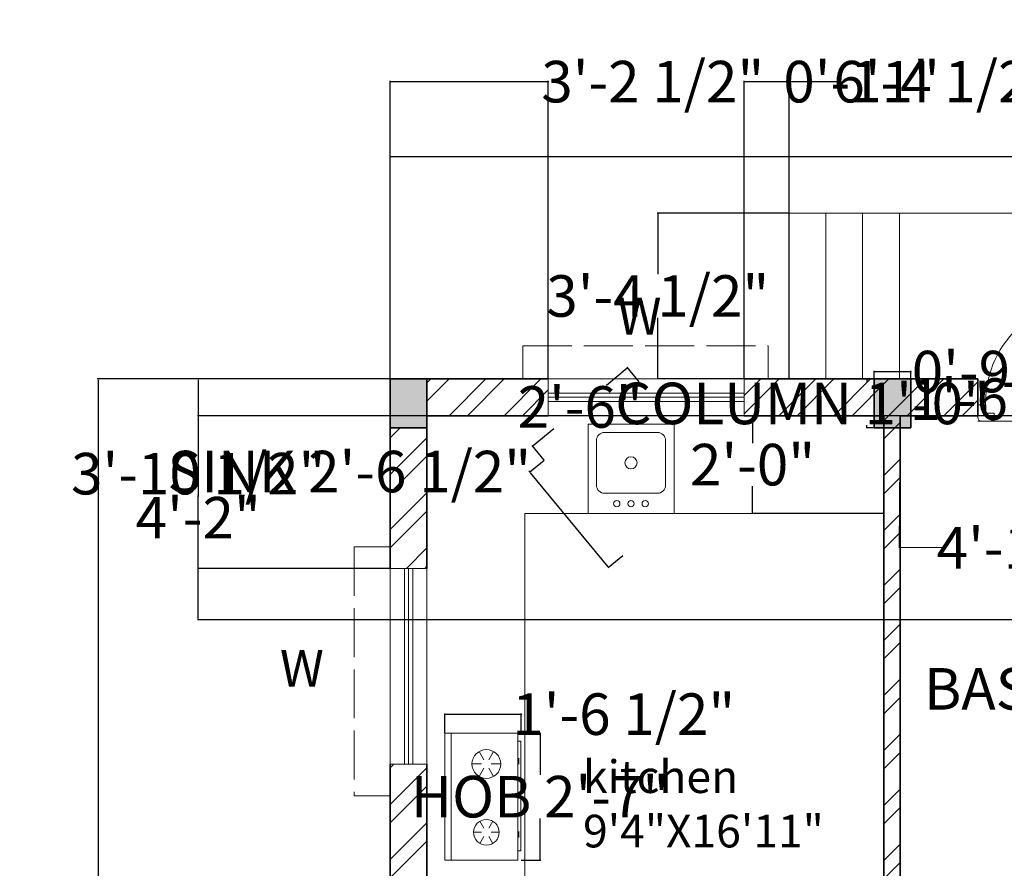
# Model space of a CAD drawing. Units: inches. Extents: x 2379 to 3013, y 1431 to 2110.
# Tile 4 of 10: x 2379 to 2620, y 1902 to 2110. Entities that reach past the tile are written whole.
import ezdxf

# ---------------------------------------------------------------- set-up
doc = ezdxf.new("R2010")
doc.units = ezdxf.units.IN
doc.linetypes.add('ACAD_ISO02W100', pattern=[15, 12, -3])
for name, color, linetype, lineweight in [('A-ANNO-DIMS', 2, 'Continuous', 18), ('A-ANNO-TEXT', 7, 'Continuous', 18), ('A-AREA-IDEN', 7, 'Continuous', 18), ('A-COLS', 7, 'Continuous', 35), ('A-COLS-PATT', 252, 'Continuous', 13), ('A-DOOR', 4, 'Continuous', 18), ('A-EQPM', 9, 'Continuous', 18), ('A-FLOR-CASE', 8, 'Continuous', 18), ('A-FLOR-FIXT', 9, 'Continuous', 18), ('A-FLOR-STRS', 7, 'Continuous', 18), ('A-ROOF-OVHD', 11, 'ACAD_ISO02W100', 13), ('A-WALL-PATT', 8, 'Continuous', 13), ('A_FUR 1', 5, 'Continuous', 5), ('A_TEXT_SMALL', 18, 'Continuous', 5), ('WALL', 7, 'Continuous', 35), ('WINDOW', 4, 'Continuous', 15)]:
    doc.layers.add(name, color=color, linetype=linetype, lineweight=lineweight)
doc.layers.add('FURN3D', color=229, linetype='Continuous', lineweight=5, true_color=0x4a3f41)
doc.styles.get("Standard").update_dxf_attribs({"font": 'arial.ttf'})
doc.dimstyles.get("Standard").update_dxf_attribs({"dimtxt": 10.18, "dimasz": 0.18, "dimexe": 0.18, "dimexo": 0.0625, "dimgap": 0.09, "dimtad": 0, "dimtih": 1, "dimtoh": 1, "dimdec": 0, "dimzin": 0, "dimdsep": 46, "dimlunit": 3, "dimtxsty": 'Standard', "dimcen": 0.09, "dimadec": 0, "dimazin": 0, "dimtfac": 1, "dimtdec": 0, "dimtofl": 0, "dimtmove": 0, "dimatfit": 3, "dimfxl": 1, "dimtolj": 1, "dimtzin": 0, "dimarcsym": 0})

# ---------------------------------------------------------------- blocks, each defined once
blk = doc.blocks.new('column')
for p, q in [((2588.21, 2021.79), (2597.21, 2021.79)), ((2588.21, 2009.79), (2588.21, 2021.79)), ((2597.21, 2021.79), (2597.21, 2009.79)), ((2597.21, 2009.79), (2588.21, 2009.79))]:
    blk.add_line(p, q)
blk = doc.blocks.new('ESTSET')
at = {"layer": 'A_FUR 1'}
for p, q in [((-10.44, 4.1), (-10.44, 32.1)), ((-8.44, 4.1), (-8.44, 32.1)), ((-36.44, 6.1), (-36.44, 3.1)), ((-34.44, 6.1), (-36.44, 6.1)), ((-34.44, 4.1), (-34.44, 6.1)), ((-34.44, 4.1), (-34.44, 6.1)), ((-8.44, 4.1), (-8.44, 6.1)), ((-8.44, 6.1), (-6.44, 6.1)), ((-8.44, 4.1), (-8.44, 6.1)), ((-6.44, 6.1), (-6.44, 3.1)), ((-32.44, 4.1), (-34.44, 4.1)), ((-32.44, 4.1), (-34.44, 4.1)), ((-32.44, 3.1), (-32.44, 4.1)), ((-10.44, 3.1), (-10.44, 4.1)), ((-10.44, 4.1), (-8.44, 4.1)), ((-10.44, 4.1), (-8.44, 4.1)), ((-6.44, 2.1), (-36.44, 2.1)), ((-35.44, 2.1), (-33.44, 2.1)), ((-7.44, 2.1), (-9.44, 2.1))]:
    blk.add_line(p, q, dxfattribs=at)
for points in [[(-21.44, 2.1), (-18.67, 2.1), (-18.67, 5.1), (-20.06, 5.1)], [(-20.06, 5.1), (-20.06, -0.91)], [(-21.44, 2.1), (-21.44, -0.91), (-20.06, -0.91)]]:
    blk.add_lwpolyline(points, dxfattribs=at)
for centre, radius, start, end in [((-8.91, 6.46), 25.64, 88.9606, 185.2816), ((-35.44, 3.1), 1, 180, 270), ((-33.44, 3.1), 1, 270, 0), ((-9.44, 3.1), 1, 180, 270), ((-7.44, 3.1), 1, 270, 0)]:
    blk.add_arc(centre, radius, start, end, dxfattribs=at)
blk = doc.blocks.new('A$C21540130')
at = {"layer": 'FURN3D'}
for p, q in [((1.57, 0), (1.57, 31.11)), ((9.61, 25.31), (8.63, 27.01)), ((10.79, 25.31), (11.77, 27.01)), ((9.02, 24.29, -27.54), (7.06, 24.29, -27.54)), ((11.38, 24.29, -27.54), (13.34, 24.29, -27.54)), ((9.61, 23.27), (8.63, 21.57)), ((10.79, 23.27), (11.77, 21.57)), ((9.61, 8.56), (8.43, 10.6)), ((10.79, 8.56), (11.97, 10.6)), ((9.02, 7.54), (6.67, 7.54)), ((11.38, 7.54), (13.73, 7.54)), ((9.61, 6.52), (8.43, 4.48)), ((10.79, 6.52), (11.97, 4.48))]:
    blk.add_line(p, q, dxfattribs=at)
for points in [[(0, 0), (0, 31.11), (17.9, 31.11), (17.9, 0)], [(18.68, 1.96), (18.68, 28.83), (17.9, 28.83), (17.9, 1.96)]]:
    blk.add_lwpolyline(points, close=True, dxfattribs=at)
for centre, radius in [((10.2, 24.29), 3.14), ((10.2, 7.54), 3.53)]:
    blk.add_circle(centre, radius, dxfattribs=at)
for points in [[(17.9, 24.03), (18.29, 24.03), (17.9, 25.6), (18.29, 25.6)], [(17.9, 6.05), (18.29, 6.05), (17.9, 7.62), (18.29, 7.62)]]:
    blk.add_solid(points, dxfattribs=at)
blk = doc.blocks.new('reh-flat-2')
at = {"layer": 'A_TEXT_SMALL'}
for p, q in [((486053827.2, -394630231.2), (486054182.4, -394629799.8)), ((486054182.4, -394629799.8), (486054596.6, -394630140.9)), ((486053979.5, -394630126.3), (486054157.1, -394629910.6)), ((486054228.6, -394629903.6), (486054483.5, -394630113.5)), ((486054596.6, -394630140.9), (486054241.4, -394630572.3)), ((486054490.4, -394630185), (486054312.8, -394630400.7)), ((486054241.4, -394630572.3), (486053827.2, -394630231.2)), ((486054241.3, -394630407.7), (486053986.4, -394630197.8))]:
    blk.add_line(p, q, dxfattribs=at)
for centre, radius in [((486054234.9, -394630155.7), 38.1), ((486054004.1, -394630296.2), 20.1), ((486054072.7, -394630352.7), 20.1), ((486054141.4, -394630409.3), 20.1)]:
    blk.add_circle(centre, radius, dxfattribs=at)
for centre, start, end in [((486054196.3, -394629942.9), 50.53053, 140.53053), ((486054018.7, -394630158.5), 140.53053, 230.53053), ((486054451.2, -394630152.8), 320.53053, 50.53053), ((486054273.6, -394630368.4), 230.53053, 320.53053)]:
    blk.add_arc(centre, 50.8, start, end, dxfattribs=at)
blk = doc.blocks.new('*D13')
at = {"layer": 'A-ANNO-DIMS', "color": 0, "lineweight": -2, "transparency": 16777216}
for p, q in [((2469.57, 2021.61), (2397.82, 2021.61)), ((2398, 2021.43), (2398, 1755.4)), ((2398, 1478.79), (2398, 1744.82)), ((2469.57, 1478.61), (2397.82, 1478.61))]:
    blk.add_line(p, q, dxfattribs=at)
at = {"layer": 'A-ANNO-DIMS', "color": 0, "transparency": 16777216}
for points in [[(2397.97, 2021.43), (2398.03, 2021.43), (2398, 2021.61)], [(2397.97, 1478.79), (2398.03, 1478.79), (2398, 1478.61)]]:
    blk.add_solid(points, dxfattribs=at)
at = {"layer": 'Defpoints', "color": 0, "transparency": 16777216}
for p in [(2469.63, 2021.61), (2398, 1478.61), (2469.63, 1478.61)]:
    blk.add_point(p, dxfattribs=at)
at = {"layer": 'A-ANNO-DIMS', "color": 0, "transparency": 16777216, "insert": (2398, 1750.11), "char_height": 10.18, "attachment_point": 5}
blk.add_mtext('\\A1;45\'-3"', dxfattribs=at)
blk = doc.blocks.new('*D14')
at = {"layer": 'A-ANNO-DIMS', "color": 0, "lineweight": -2, "transparency": 16777216}
for p, q in [((2469.63, 2021.67), (2469.63, 2076.34)), ((2469.81, 2076.16), (2694.9, 2076.16)), ((2937.45, 2076.16), (2712.35, 2076.16)), ((2937.63, 2021.67), (2937.63, 2076.34))]:
    blk.add_line(p, q, dxfattribs=at)
at = {"layer": 'A-ANNO-DIMS', "color": 0, "transparency": 16777216}
for points in [[(2469.81, 2076.19), (2469.81, 2076.13), (2469.63, 2076.16)], [(2937.45, 2076.19), (2937.45, 2076.13), (2937.63, 2076.16)]]:
    blk.add_solid(points, dxfattribs=at)
at = {"layer": 'Defpoints', "color": 0, "transparency": 16777216}
for p in [(2937.63, 2076.16), (2469.63, 2021.61), (2937.63, 2021.61)]:
    blk.add_point(p, dxfattribs=at)
at = {"layer": 'A-ANNO-DIMS', "color": 0, "transparency": 16777216, "insert": (2703.63, 2076.16), "char_height": 10.18, "attachment_point": 5}
blk.add_mtext("\\A1;39'", dxfattribs=at)
blk = doc.blocks.new('WIN-48IN')
for p, q in [((0, 48), (0, 0)), ((9, 48), (0, 48)), ((3.5, 48), (3.5, 0)), ((4.5, 48), (4.5, 0)), ((5.5, 48), (5.5, 0)), ((9, 0), (9, 48)), ((9, 0), (0, 0))]:
    blk.add_line(p, q)
blk = doc.blocks.new('*D20')
at = {"layer": 'A-ANNO-DIMS', "color": 0, "lineweight": -2, "transparency": 16777216}
for p, q in [((2588.15, 2021.61), (2586.23, 2021.61)), ((2586.41, 2021.43), (2586.41, 2020.97)), ((2586.41, 2009.79), (2586.41, 2010.25)), ((2588.15, 2009.61), (2586.23, 2009.61))]:
    blk.add_line(p, q, dxfattribs=at)
at = {"layer": 'A-ANNO-DIMS', "color": 0, "transparency": 16777216}
for points in [[(2586.38, 2021.43), (2586.44, 2021.43), (2586.41, 2021.61)], [(2586.38, 2009.79), (2586.44, 2009.79), (2586.41, 2009.61)]]:
    blk.add_solid(points, dxfattribs=at)
at = {"layer": 'Defpoints', "color": 0, "transparency": 16777216}
for p in [(2586.41, 2021.61), (2588.21, 2021.61), (2588.21, 2009.61)]:
    blk.add_point(p, dxfattribs=at)
at = {"layer": 'A-ANNO-DIMS', "color": 0, "transparency": 16777216, "insert": (2586.41, 2015.61), "char_height": 10.18, "attachment_point": 5}
blk.add_mtext('\\A1;COLUMN 1\'-0" TYP.', dxfattribs=at)
blk = doc.blocks.new('*D21')
at = {"layer": 'A-ANNO-DIMS', "color": 0, "lineweight": -2, "transparency": 16777216}
for p, q in [((2588.21, 2021.67), (2588.21, 2023.59)), ((2588.39, 2023.41), (2597.03, 2023.41)), ((2597.21, 2021.67), (2597.21, 2023.59)), ((2597.21, 2023.41), (2597.39, 2023.41))]:
    blk.add_line(p, q, dxfattribs=at)
at = {"layer": 'A-ANNO-DIMS', "color": 0, "transparency": 16777216}
for points in [[(2588.39, 2023.44), (2588.39, 2023.38), (2588.21, 2023.41)], [(2597.03, 2023.44), (2597.03, 2023.38), (2597.21, 2023.41)]]:
    blk.add_solid(points, dxfattribs=at)
at = {"layer": 'Defpoints', "color": 0, "transparency": 16777216}
for p in [(2597.21, 2023.41), (2588.21, 2021.61), (2597.21, 2021.61)]:
    blk.add_point(p, dxfattribs=at)
at = {"layer": 'A-ANNO-DIMS', "color": 0, "transparency": 16777216, "insert": (2628.51, 2023.41), "char_height": 10.18, "attachment_point": 5}
blk.add_mtext('\\A1;0\'-9" TYP.', dxfattribs=at)
blk = doc.blocks.new('*D38')
at = {"layer": 'A-ANNO-DIMS', "color": 0, "lineweight": -2, "transparency": 16777216}
for p, q in [((2501.74, 1934.8), (2506.52, 1934.8)), ((2506.34, 1934.62), (2506.34, 1924.61)), ((2506.34, 1903.88), (2506.34, 1913.89)), ((2501.74, 1903.7), (2506.52, 1903.7))]:
    blk.add_line(p, q, dxfattribs=at)
at = {"layer": 'A-ANNO-DIMS', "color": 0, "transparency": 16777216}
for points in [[(2506.31, 1934.62), (2506.37, 1934.62), (2506.34, 1934.8)], [(2506.31, 1903.88), (2506.37, 1903.88), (2506.34, 1903.7)]]:
    blk.add_solid(points, dxfattribs=at)
at = {"layer": 'Defpoints', "color": 0, "transparency": 16777216}
for p in [(2501.68, 1934.8), (2501.68, 1903.7), (2506.34, 1903.7)]:
    blk.add_point(p, dxfattribs=at)
at = {"layer": 'A-ANNO-DIMS', "color": 0, "transparency": 16777216, "insert": (2506.34, 1919.25), "char_height": 10.18, "attachment_point": 5}
blk.add_mtext('\\A1;HOB 2\'-7"', dxfattribs=at)
blk = doc.blocks.new('*D39')
at = {"layer": 'A-ANNO-DIMS', "color": 0, "lineweight": -2, "transparency": 16777216}
for p, q in [((2482.99, 1934.86), (2482.99, 1939.65)), ((2483.17, 1939.47), (2501.5, 1939.47)), ((2501.68, 1934.86), (2501.68, 1939.65)), ((2501.68, 1939.47), (2501.86, 1939.47))]:
    blk.add_line(p, q, dxfattribs=at)
at = {"layer": 'A-ANNO-DIMS', "color": 0, "transparency": 16777216}
for points in [[(2483.17, 1939.5), (2483.17, 1939.44), (2482.99, 1939.47)], [(2501.5, 1939.5), (2501.5, 1939.44), (2501.68, 1939.47)]]:
    blk.add_solid(points, dxfattribs=at)
at = {"layer": 'Defpoints', "color": 0, "transparency": 16777216}
for p in [(2501.68, 1939.47), (2482.99, 1934.8), (2501.68, 1934.8)]:
    blk.add_point(p, dxfattribs=at)
at = {"layer": 'A-ANNO-DIMS', "color": 0, "transparency": 16777216, "insert": (2526.86, 1939.47), "char_height": 10.18, "attachment_point": 5}
blk.add_mtext('\\A1;1\'-6 1/2"', dxfattribs=at)
blk = doc.blocks.new('*D41')
at = {"layer": 'A-ANNO-DIMS', "color": 0, "lineweight": -2, "transparency": 16777216}
for p, q in [((2658.82, 2016.68), (2658.64, 2016.68)), ((2658.82, 2012.67), (2658.82, 2016.86)), ((2676.75, 2016.68), (2659, 2016.68)), ((2676.93, 2012.67), (2676.93, 2016.86))]:
    blk.add_line(p, q, dxfattribs=at)
at = {"layer": 'A-ANNO-DIMS', "color": 0, "transparency": 16777216}
for points in [[(2659, 2016.71), (2659, 2016.65), (2658.82, 2016.68)], [(2676.75, 2016.71), (2676.75, 2016.65), (2676.93, 2016.68)]]:
    blk.add_solid(points, dxfattribs=at)
at = {"layer": 'Defpoints', "color": 0, "transparency": 16777216}
for p in [(2658.82, 2016.68), (2658.82, 2012.61), (2676.93, 2012.61)]:
    blk.add_point(p, dxfattribs=at)
at = {"layer": 'A-ANNO-DIMS', "color": 0, "transparency": 16777216, "insert": (2628, 2016.68), "char_height": 10.18, "attachment_point": 5}
blk.add_mtext('\\A1;1\'-6" TYP.', dxfattribs=at)
blk = doc.blocks.new('*D42')
at = {"layer": 'A-ANNO-DIMS', "color": 0, "lineweight": -2, "transparency": 16777216}
for p, q in [((2731.29, 1945.67), (2731.11, 1945.67)), ((2731.29, 1942.77), (2731.29, 1945.85)), ((2750.86, 1945.67), (2731.47, 1945.67)), ((2751.04, 1942.77), (2751.04, 1945.85))]:
    blk.add_line(p, q, dxfattribs=at)
at = {"layer": 'A-ANNO-DIMS', "color": 0, "transparency": 16777216}
for points in [[(2731.47, 1945.7), (2731.47, 1945.64), (2731.29, 1945.67)], [(2750.86, 1945.7), (2750.86, 1945.64), (2751.04, 1945.67)]]:
    blk.add_solid(points, dxfattribs=at)
at = {"layer": 'Defpoints', "color": 0, "transparency": 16777216}
for p in [(2731.29, 1945.67), (2731.29, 1942.71), (2751.04, 1942.71)]:
    blk.add_point(p, dxfattribs=at)
at = {"layer": 'A-ANNO-DIMS', "color": 0, "transparency": 16777216, "insert": (2665.05, 1945.67), "char_height": 10.18, "attachment_point": 5}
blk.add_mtext('\\A1;BASIN 1\'-7 1/2" TYP.', dxfattribs=at)
blk = doc.blocks.new('*D44')
at = {"layer": 'A-ANNO-DIMS', "color": 0, "lineweight": -2, "transparency": 16777216}
for p, q in [((2507.38, 2001.62), (2503.78, 1998.66)), ((2503.81, 1998.91), (2503.63, 1998.91)), ((2503.92, 1998.77), (2503.81, 1998.91)), ((2523.05, 1975.54), (2504.04, 1998.64)), ((2526.62, 1978.25), (2523.03, 1975.29))]:
    blk.add_line(p, q, dxfattribs=at)
at = {"layer": 'A-ANNO-DIMS', "color": 0, "transparency": 16777216}
for points in [[(2504.06, 1998.65), (2504.01, 1998.62), (2503.92, 1998.77)], [(2523.08, 1975.56), (2523.03, 1975.52), (2523.17, 1975.4)]]:
    blk.add_solid(points, dxfattribs=at)
at = {"layer": 'Defpoints', "color": 0, "transparency": 16777216}
for p in [(2507.43, 2001.66), (2503.92, 1998.77), (2526.67, 1978.29)]:
    blk.add_point(p, dxfattribs=at)
at = {"layer": 'A-ANNO-DIMS', "color": 0, "transparency": 16777216, "insert": (2459.6, 1998.91), "char_height": 10.18, "attachment_point": 5}
blk.add_mtext('\\A1;SINK 2\'-6 1/2"', dxfattribs=at)
blk = doc.blocks.new('*D45')
at = {"layer": 'A-ANNO-DIMS', "color": 0, "lineweight": -2, "transparency": 16777216}
for p, q in [((2527.68, 2024.22), (2522.6, 2020.04)), ((2530.67, 2020.88), (2527.71, 2024.48)), ((2504.68, 2005.28), (2509.76, 2009.47)), ((2507.39, 2001.71), (2504.43, 2005.31))]:
    blk.add_line(p, q, dxfattribs=at)
at = {"layer": 'A-ANNO-DIMS', "color": 0, "transparency": 16777216}
for points in [[(2527.66, 2024.25), (2527.7, 2024.2), (2527.82, 2024.34)], [(2504.66, 2005.3), (2504.7, 2005.26), (2504.54, 2005.17)]]:
    blk.add_solid(points, dxfattribs=at)
at = {"layer": 'Defpoints', "color": 0, "transparency": 16777216}
for p in [(2527.82, 2024.34), (2530.71, 2020.83), (2507.43, 2001.66)]:
    blk.add_point(p, dxfattribs=at)
at = {"layer": 'A-ANNO-DIMS', "color": 0, "transparency": 16777216, "insert": (2516.18, 2014.75), "char_height": 10.18, "attachment_point": 5}
blk.add_mtext('\\A1;2\'-6"', dxfattribs=at)
blk = doc.blocks.new('*D51')
at = {"layer": 'A-ANNO-DIMS', "color": 0, "lineweight": -2, "transparency": 16777216}
for p, q in [((2567.4, 2062.32), (2567.4, 2094.64)), ((2567.58, 2094.46), (2580.04, 2094.46)), ((2643.52, 2094.46), (2631.06, 2094.46)), ((2643.7, 2062.32), (2643.7, 2094.64))]:
    blk.add_line(p, q, dxfattribs=at)
at = {"layer": 'A-ANNO-DIMS', "color": 0, "transparency": 16777216}
for points in [[(2567.58, 2094.49), (2567.58, 2094.43), (2567.4, 2094.46)], [(2643.52, 2094.49), (2643.52, 2094.43), (2643.7, 2094.46)]]:
    blk.add_solid(points, dxfattribs=at)
at = {"layer": 'Defpoints', "color": 0, "transparency": 16777216}
for p in [(2643.7, 2094.46), (2567.4, 2062.26), (2643.7, 2062.26)]:
    blk.add_point(p, dxfattribs=at)
at = {"layer": 'A-ANNO-DIMS', "color": 0, "transparency": 16777216, "insert": (2605.55, 2094.46), "char_height": 10.18, "attachment_point": 5}
blk.add_mtext('\\A1;6\'-4 1/2"', dxfattribs=at)
blk = doc.blocks.new('*D52')
at = {"layer": 'A-ANNO-DIMS', "color": 0, "lineweight": -2, "transparency": 16777216}
for p, q in [((2567.33, 2062.26), (2535.02, 2062.26)), ((2535.2, 2062.08), (2535.2, 2047.29)), ((2535.2, 2021.79), (2535.2, 2036.58)), ((2567.33, 2021.61), (2535.02, 2021.61))]:
    blk.add_line(p, q, dxfattribs=at)
at = {"layer": 'A-ANNO-DIMS', "color": 0, "transparency": 16777216}
for points in [[(2535.17, 2062.08), (2535.23, 2062.08), (2535.2, 2062.26)], [(2535.17, 2021.79), (2535.23, 2021.79), (2535.2, 2021.61)]]:
    blk.add_solid(points, dxfattribs=at)
at = {"layer": 'Defpoints', "color": 0, "transparency": 16777216}
for p in [(2535.2, 2062.26), (2567.4, 2062.26), (2567.4, 2021.61)]:
    blk.add_point(p, dxfattribs=at)
at = {"layer": 'A-ANNO-DIMS', "color": 0, "transparency": 16777216, "insert": (2535.2, 2041.94), "char_height": 10.18, "attachment_point": 5}
blk.add_mtext('\\A1;3\'-4 1/2"', dxfattribs=at)
blk = doc.blocks.new('*D56')
at = {"layer": 'A-ANNO-DIMS', "color": 0, "lineweight": -2, "transparency": 16777216}
for p, q in [((2647.57, 2012.61), (2422.39, 2012.61)), ((2422.57, 2012.43), (2422.57, 1992.81)), ((2422.57, 1962.79), (2422.57, 1982.41)), ((2647.57, 1962.61), (2422.39, 1962.61))]:
    blk.add_line(p, q, dxfattribs=at)
at = {"layer": 'A-ANNO-DIMS', "color": 0, "transparency": 16777216}
for points in [[(2422.54, 2012.43), (2422.6, 2012.43), (2422.57, 2012.61)], [(2422.54, 1962.79), (2422.6, 1962.79), (2422.57, 1962.61)]]:
    blk.add_solid(points, dxfattribs=at)
at = {"layer": 'Defpoints', "color": 0, "transparency": 16777216}
for p in [(2647.63, 2012.61), (2422.57, 1962.61), (2647.63, 1962.61)]:
    blk.add_point(p, dxfattribs=at)
at = {"layer": 'A-ANNO-DIMS', "color": 0, "transparency": 16777216, "insert": (2422.57, 1987.61), "char_height": 10.18, "attachment_point": 5}
blk.add_mtext('\\A1;4\'-2"', dxfattribs=at)
blk = doc.blocks.new('*D58')
at = {"layer": 'A-ANNO-DIMS', "color": 0, "lineweight": -2, "transparency": 16777216}
for p, q in [((2469.57, 2021.61), (2422.39, 2021.61)), ((2422.57, 2021.43), (2422.57, 2003.76)), ((2422.57, 1975.37), (2422.57, 1993.04)), ((2469.57, 1975.19), (2422.39, 1975.19))]:
    blk.add_line(p, q, dxfattribs=at)
at = {"layer": 'A-ANNO-DIMS', "color": 0, "transparency": 16777216}
for points in [[(2422.54, 2021.43), (2422.6, 2021.43), (2422.57, 2021.61)], [(2422.54, 1975.37), (2422.6, 1975.37), (2422.57, 1975.19)]]:
    blk.add_solid(points, dxfattribs=at)
at = {"layer": 'Defpoints', "color": 0, "transparency": 16777216}
for p in [(2422.57, 2021.61), (2469.63, 2021.61), (2469.63, 1975.19)]:
    blk.add_point(p, dxfattribs=at)
at = {"layer": 'A-ANNO-DIMS', "color": 0, "transparency": 16777216, "insert": (2422.57, 1998.4), "char_height": 10.18, "attachment_point": 5}
blk.add_mtext('\\A1;3\'-10 1/2"', dxfattribs=at)
blk = doc.blocks.new('*D59')
at = {"layer": 'A-ANNO-DIMS', "color": 0, "lineweight": -2, "transparency": 16777216}
for p, q in [((2469.63, 2021.67), (2469.63, 2094.64)), ((2469.81, 2094.46), (2508.15, 2094.46)), ((2508.33, 2021.67), (2508.33, 2094.64)), ((2508.33, 2094.46), (2508.51, 2094.46))]:
    blk.add_line(p, q, dxfattribs=at)
at = {"layer": 'A-ANNO-DIMS', "color": 0, "transparency": 16777216}
for points in [[(2469.81, 2094.49), (2469.81, 2094.43), (2469.63, 2094.46)], [(2508.15, 2094.49), (2508.15, 2094.43), (2508.33, 2094.46)]]:
    blk.add_solid(points, dxfattribs=at)
at = {"layer": 'Defpoints', "color": 0, "transparency": 16777216}
for p in [(2508.33, 2094.46), (2469.63, 2021.61), (2508.33, 2021.61)]:
    blk.add_point(p, dxfattribs=at)
at = {"layer": 'A-ANNO-DIMS', "color": 0, "transparency": 16777216, "insert": (2533.98, 2094.46), "char_height": 10.18, "attachment_point": 5}
blk.add_mtext('\\A1;3\'-2 1/2"', dxfattribs=at)
blk = doc.blocks.new('*D67')
at = {"layer": 'A-ANNO-DIMS', "color": 0, "lineweight": -2, "transparency": 16777216}
for p, q in [((2590.57, 2012.61), (2558.25, 2012.61)), ((2558.43, 2012.43), (2558.43, 2005.9)), ((2558.43, 1988.79), (2558.43, 1995.32)), ((2590.57, 1988.61), (2558.25, 1988.61))]:
    blk.add_line(p, q, dxfattribs=at)
at = {"layer": 'A-ANNO-DIMS', "color": 0, "transparency": 16777216}
for points in [[(2558.4, 2012.43), (2558.46, 2012.43), (2558.43, 2012.61)], [(2558.4, 1988.79), (2558.46, 1988.79), (2558.43, 1988.61)]]:
    blk.add_solid(points, dxfattribs=at)
at = {"layer": 'Defpoints', "color": 0, "transparency": 16777216}
for p in [(2558.43, 2012.61), (2590.63, 2012.61), (2590.63, 1988.61)]:
    blk.add_point(p, dxfattribs=at)
at = {"layer": 'A-ANNO-DIMS', "color": 0, "transparency": 16777216, "insert": (2558.43, 2000.61), "char_height": 10.18, "attachment_point": 5}
blk.add_mtext('\\A1;2\'-0"', dxfattribs=at)
blk = doc.blocks.new('*D68')
at = {"layer": 'A-ANNO-DIMS', "color": 0, "lineweight": -2, "transparency": 16777216}
for p, q in [((2556.33, 2021.67), (2556.33, 2094.64)), ((2556.51, 2094.46), (2567.22, 2094.46)), ((2567.4, 2021.67), (2567.4, 2094.64)), ((2567.4, 2094.46), (2567.58, 2094.46))]:
    blk.add_line(p, q, dxfattribs=at)
at = {"layer": 'A-ANNO-DIMS', "color": 0, "transparency": 16777216}
for points in [[(2556.51, 2094.49), (2556.51, 2094.43), (2556.33, 2094.46)], [(2567.22, 2094.49), (2567.22, 2094.43), (2567.4, 2094.46)]]:
    blk.add_solid(points, dxfattribs=at)
at = {"layer": 'Defpoints', "color": 0, "transparency": 16777216}
for p in [(2567.4, 2094.46), (2556.33, 2021.61), (2567.4, 2021.61)]:
    blk.add_point(p, dxfattribs=at)
at = {"layer": 'A-ANNO-DIMS', "color": 0, "transparency": 16777216, "insert": (2585.15, 2094.46), "char_height": 10.18, "attachment_point": 5}
blk.add_mtext('\\A1;0\'-11"', dxfattribs=at)
blk = doc.blocks.new('*D70')
at = {"layer": 'A-ANNO-DIMS', "color": 0, "lineweight": -2, "transparency": 16777216}
for p, q in [((2594.63, 2012.55), (2594.39, 1980.23)), ((2643.63, 2012.19), (2643.39, 1979.87)), ((2594.57, 1980.41), (2605.07, 1980.33)), ((2643.21, 1980.05), (2632.72, 1980.13))]:
    blk.add_line(p, q, dxfattribs=at)
at = {"layer": 'A-ANNO-DIMS', "color": 0, "transparency": 16777216}
for points in [[(2594.57, 1980.44), (2594.57, 1980.38), (2594.39, 1980.41)], [(2643.21, 1980.08), (2643.21, 1980.02), (2643.39, 1980.05)]]:
    blk.add_solid(points, dxfattribs=at)
at = {"layer": 'Defpoints', "color": 0, "transparency": 16777216}
for p in [(2594.63, 2012.61), (2643.63, 2012.25), (2594.39, 1980.41)]:
    blk.add_point(p, dxfattribs=at)
at = {"layer": 'A-ANNO-DIMS', "color": 0, "transparency": 16777216, "insert": (2618.89, 1980.23), "char_height": 10.18, "attachment_point": 5}
blk.add_mtext('\\A1;4\'-1"', dxfattribs=at)

msp = doc.modelspace()

# ---------------------------------------------------------------- hatches: boundary and pattern name
at = {"layer": 'A-COLS-PATT'}
h = msp.add_hatch(color=256, dxfattribs=at)
h.dxf.hatch_style = 1
h.paths.add_polyline_path([(2478.63, 2021.61), (2469.63, 2021.61), (2469.63, 2009.61), (2478.63, 2009.61)])
h = msp.add_hatch(color=256, dxfattribs=at)
h.dxf.hatch_style = 1
h.paths.add_polyline_path([(2937.62, 1660.61), (2925.62, 1660.61), (2925.62, 1651.61), (2937.62, 1651.61)])
h.paths.add_polyline_path([(2481.63, 1809.61), (2478.63, 1809.61), (2478.63, 1811.02), (2469.63, 1811.02), (2469.63, 1802.02), (2478.63, 1802.02), (2478.63, 1805.61), (2481.63, 1805.61)])
h.paths.add_polyline_path([(2481.63, 1811.02), (2478.63, 1811.02), (2478.63, 1809.61), (2481.63, 1809.61)], flags=17)
h.paths.add_polyline_path([(2481.63, 1805.61), (2478.63, 1805.61), (2478.63, 1802.02), (2481.63, 1802.02)], flags=17)
h.paths.add_polyline_path([(2481.63, 1660.61), (2469.63, 1660.61), (2469.63, 1651.61), (2481.63, 1651.61)])
h.paths.add_polyline_path([(2692.07, 1660.61), (2688.63, 1660.61), (2688.63, 1663.61), (2684.63, 1663.61), (2684.63, 1660.61), (2683.07, 1660.61), (2683.07, 1651.61), (2692.07, 1651.61)])
h.paths.add_polyline_path([(2692.07, 1663.61), (2688.63, 1663.61), (2688.63, 1660.61), (2692.07, 1660.61)], flags=17)
h.paths.add_polyline_path([(2684.63, 1663.61), (2683.07, 1663.61), (2683.07, 1660.61), (2684.63, 1660.61)], flags=17)
h.paths.add_polyline_path([(2770.63, 1660.61), (2767.63, 1660.61), (2767.63, 1663.61), (2763.63, 1663.61), (2763.63, 1660.61), (2761.63, 1660.61), (2761.63, 1651.61), (2763.63, 1651.61), (2767.63, 1651.61), (2767.63, 1651.61), (2770.63, 1651.61)])
h.paths.add_polyline_path([(2770.63, 1663.61), (2767.63, 1663.61), (2767.63, 1660.61), (2770.63, 1660.61)], flags=17)
h.paths.add_polyline_path([(2763.63, 1663.61), (2761.63, 1663.61), (2761.63, 1660.61), (2763.63, 1660.61)], flags=17)
h.paths.add_polyline_path([(2937.63, 1813.62), (2928.63, 1813.62), (2928.63, 1810.61), (2925.63, 1810.61), (2925.63, 1806.61), (2928.63, 1806.61), (2928.63, 1804.62), (2937.63, 1804.62)], flags=17)
h.paths.add_polyline_path([(2937.63, 1813.62), (2928.63, 1813.62), (2928.63, 1810.61), (2925.63, 1810.61), (2925.63, 1804.62), (2937.63, 1804.62)], flags=17)
h.paths.add_polyline_path([(2928.63, 1813.62), (2925.63, 1813.62), (2925.63, 1810.61), (2928.63, 1810.61)], flags=0)
h.paths.add_polyline_path([(2937.63, 1863.8), (2928.63, 1863.8), (2928.63, 1862.61), (2925.63, 1862.61), (2925.63, 1858.61), (2928.63, 1858.61), (2928.63, 1854.8), (2937.63, 1854.8)])
h.paths.add_polyline_path([(2928.63, 1863.8), (2925.63, 1863.8), (2925.63, 1862.61), (2928.63, 1862.61)], flags=17)
h.paths.add_polyline_path([(2928.63, 1858.61), (2925.63, 1858.61), (2925.63, 1854.8), (2928.63, 1854.8)], flags=17)
h.paths.add_polyline_path([(2937.63, 2021.61), (2928.63, 2021.61), (2928.63, 2012.61), (2928.63, 2012.61), (2928.63, 2009.61), (2937.63, 2009.61)])
h.paths.add_polyline_path([(2770.27, 2021.61), (2761.27, 2021.61), (2761.27, 2012.61), (2763.63, 2012.61), (2763.63, 2009.61), (2767.63, 2009.61), (2767.63, 2012.61), (2770.27, 2012.61)])
h.paths.add_polyline_path([(2763.63, 2012.61), (2761.27, 2012.61), (2761.27, 2009.61), (2763.63, 2009.61)], flags=17)
h.paths.add_polyline_path([(2770.27, 2012.61), (2767.63, 2012.61), (2767.63, 2009.61), (2770.27, 2009.61)], flags=17)
h.paths.add_polyline_path([(2597.21, 2021.61), (2588.21, 2021.61), (2588.21, 2012.61), (2590.63, 2012.61), (2590.63, 2009.61), (2594.63, 2009.61), (2594.63, 2012.61), (2597.21, 2012.61)])
h.paths.add_polyline_path([(2590.63, 2012.61), (2588.21, 2012.61), (2588.21, 2009.61), (2590.63, 2009.61)], flags=17)
h.paths.add_polyline_path([(2597.21, 2012.61), (2594.63, 2012.61), (2594.63, 2009.61), (2597.21, 2009.61)], flags=17)
at = {"layer": 'A-WALL-PATT'}
h = msp.add_hatch(dxfattribs=at)
h.set_pattern_fill('ANSI32', color=256)
h.paths.add_polyline_path([(2925.63, 1862.61), (2815.63, 1862.61), (2815.63, 1858.61), (2827.63, 1858.61), (2827.63, 1810.61), (2815.63, 1810.61), (2815.63, 1806.61), (2850.78, 1806.61), (2850.78, 1810.61), (2831.63, 1810.61), (2831.63, 1858.61), (2925.63, 1858.61)])
h.paths.add_polyline_path([(2925.63, 1810.61), (2880.78, 1810.61), (2880.78, 1806.61), (2925.63, 1806.61)], flags=17)
h.paths.add_polyline_path([(2633.75, 1660.61), (2594.63, 1660.61), (2481.63, 1660.61), (2481.63, 1651.61), (2588.63, 1651.61), (2588.63, 1570.61), (2624.28, 1570.61), (2624.28, 1574.61), (2592.63, 1574.61), (2592.63, 1651.61), (2633.75, 1651.61)])
h.paths.add_polyline_path([(2594.63, 1809.61), (2481.63, 1809.61), (2481.63, 1805.61), (2594.63, 1805.61)])
h.paths.add_polyline_path([(2594.63, 2012.61), (2597.21, 2012.61), (2597.21, 2021.61), (2588.21, 2021.61), (2588.21, 2012.61), (2590.63, 2012.61), (2590.63, 1845.61), (2594.63, 1845.61)])
h.paths.add_polyline_path([(2767.63, 2012.61), (2770.27, 2012.61), (2770.27, 2021.61), (2761.27, 2021.61), (2761.27, 2012.61), (2763.63, 2012.61), (2763.63, 1928.61), (2691.63, 1928.61), (2643.63, 1928.61), (2643.63, 1924.61), (2691.63, 1924.61), (2763.63, 1924.61), (2763.63, 1858.61), (2779.63, 1858.61), (2779.63, 1862.61), (2767.63, 1862.61)])
h.paths.add_polyline_path([(2613.63, 2012.61), (2613.63, 2021.61), (2597.21, 2021.61), (2597.21, 2012.61)])
h.paths.add_polyline_path([(2508.33, 2012.61), (2508.33, 2021.61), (2478.63, 2021.61), (2478.63, 2012.61)])
h.paths.add_polyline_path([(2556.33, 2021.61), (2556.33, 2012.61), (2588.21, 2012.61), (2588.21, 2021.61)])
h.paths.add_polyline_path([(2659.15, 2012.61), (2659.15, 2021.61), (2643.63, 2021.61), (2643.63, 1958.61), (2661.63, 1958.61), (2661.63, 1962.61), (2647.63, 1962.61), (2647.63, 2012.61)])
h.paths.add_polyline_path([(2714.17, 2012.61), (2714.17, 2021.61), (2683.15, 2021.61), (2683.15, 2012.61), (2691.63, 2012.61), (2691.63, 1958.61), (2695.63, 1958.61), (2695.63, 2012.61)])
h.paths.add_polyline_path([(2738.17, 2021.61), (2738.17, 2012.61), (2761.27, 2012.61), (2761.27, 2021.61)])
h.paths.add_polyline_path([(2820.76, 2012.61), (2820.76, 2021.61), (2770.27, 2021.61), (2770.27, 2012.61)])
h.paths.add_polyline_path([(2868.76, 2021.61), (2868.76, 2012.61), (2928.63, 2012.61), (2928.63, 2021.61)])
h.paths.add_polyline_path([(2928.63, 1962.9), (2937.63, 1962.9), (2937.63, 2009.61), (2928.63, 2009.61)])
h.paths.add_polyline_path([(2937.63, 1914.9), (2928.63, 1914.9), (2928.63, 1863.8), (2937.63, 1863.8)])
h.paths.add_polyline_path([(2928.63, 1846.59), (2937.63, 1846.59), (2937.63, 1854.8), (2928.63, 1854.8)])
h.paths.add_polyline_path([(2937.63, 1822.59), (2928.63, 1822.59), (2928.63, 1813.62), (2937.63, 1813.62)])
h.paths.add_polyline_path([(2928.63, 1778.48), (2937.63, 1778.48), (2937.63, 1813.62), (2928.63, 1813.62), (2928.63, 1810.61), (2925.63, 1810.61), (2925.63, 1806.61), (2928.63, 1806.61)])
h.paths.add_polyline_path([(2816.22, 1651.61), (2816.22, 1660.61), (2767.63, 1660.61), (2767.63, 1806.61), (2779.63, 1806.61), (2779.63, 1810.61), (2763.63, 1810.61), (2763.63, 1660.61), (2688.63, 1660.61), (2688.63, 1810.61), (2684.63, 1810.61), (2684.63, 1660.61), (2669.75, 1660.61), (2669.75, 1651.61), (2763.63, 1651.61), (2763.63, 1574.61), (2672.28, 1574.61), (2672.28, 1570.61), (2767.63, 1570.61), (2767.63, 1651.61)])
h.paths.add_polyline_path([(2864.22, 1660.61), (2864.22, 1651.61), (2937.63, 1651.61), (2937.63, 1730.48), (2928.63, 1730.48), (2928.63, 1660.61)])
h.paths.add_polyline_path([(2469.63, 1975.19), (2478.63, 1975.19), (2478.63, 2009.61), (2469.63, 2009.61)])
h.paths.add_polyline_path([(2478.63, 1927.19), (2469.63, 1927.19), (2469.63, 1811.02), (2478.63, 1811.02)])
h.paths.add_polyline_path([(2469.63, 1758.04), (2478.63, 1758.04), (2478.63, 1802.02), (2469.63, 1802.02)])
h.paths.add_polyline_path([(2478.63, 1710.04), (2469.63, 1710.04), (2469.63, 1660.61), (2478.63, 1660.61)])

# ---------------------------------------------------------------- linework, layer by layer
at = {"layer": 'A-COLS'}
for p, q in [((2478.63, 2021.61), (2469.63, 2021.61)), ((2469.63, 2021.61), (2469.63, 2009.61)), ((2478.63, 2009.61), (2478.63, 2021.61)), ((2469.63, 2009.61), (2478.63, 2009.61))]:
    msp.add_line(p, q, dxfattribs=at)
at = {"layer": 'A-FLOR-CASE'}
for p, q in [((2502.63, 1809.61), (2502.63, 1988.61)), ((2502.63, 1988.61), (2590.63, 1988.61))]:
    msp.add_line(p, q, dxfattribs=at)
at = {"layer": 'A-FLOR-STRS'}
for p, q in [((2643.7, 2062.26), (2567.4, 2062.26)), ((2567.4, 2062.26), (2567.4, 2021.61)), ((2576.4, 2062.26), (2576.4, 2021.61)), ((2585.4, 2062.26), (2585.4, 2021.61)), ((2594.4, 2062.26), (2594.4, 2021.61))]:
    msp.add_line(p, q, dxfattribs=at)
at = {"layer": 'A-ROOF-OVHD'}
for p, q in [((2502.11, 2021.61), (2502.11, 2029.73)), ((2502.11, 2029.73), (2562.26, 2029.73)), ((2562.26, 2029.73), (2562.26, 2021.61)), ((2469.63, 1980.45), (2460.81, 1980.45)), ((2460.81, 1980.45), (2460.81, 1919.48)), ((2460.81, 1919.48), (2469.63, 1919.48))]:
    msp.add_line(p, q, dxfattribs=at)
at = {"layer": 'WALL'}
for p, q in [((2469.63, 2021.61), (2508.33, 2021.61)), ((2469.63, 1975.19), (2469.63, 2021.61)), ((2556.33, 2021.61), (2613.63, 2021.61)), ((2613.63, 2021.61), (2613.63, 2012.61)), ((2478.63, 2012.61), (2508.33, 2012.61)), ((2478.63, 1975.19), (2478.63, 2012.61)), ((2556.33, 2012.61), (2590.63, 2012.61)), ((2590.63, 1845.61), (2590.63, 2012.61)), ((2594.63, 2012.61), (2613.63, 2012.61)), ((2594.63, 1845.61), (2594.63, 2012.61)), ((2469.63, 1758.04), (2469.63, 1927.19)), ((2478.63, 1809.61), (2478.63, 1927.19))]:
    msp.add_line(p, q, dxfattribs=at)

# ---------------------------------------------------------------- block references
at = {"layer": 'A-COLS'}
for p in [(-118.58, -0.18), (0, -0.18)]:
    msp.add_blockref('column', p, dxfattribs=at)
at = {"layer": 'A-DOOR'}
msp.add_blockref('ESTSET', (2650.07, 2009.15), dxfattribs=at)
at = {"layer": 'A-EQPM', "xscale": -1, "rotation": 180}
msp.add_blockref('A$C21540130', (2482.99, 1934.8), dxfattribs=at)
at = {"layer": 'A-FLOR-FIXT', "xscale": 0.0391972730482577, "yscale": 0.0391972730482577, "zscale": 0.0391972730482577, "rotation": 39.46947596224971}
msp.add_blockref('reh-flat-2', (-24537686.1, -167670.17), dxfattribs=at)
at = {"layer": 'WINDOW', "rotation": 269.9999985709203}
msp.add_blockref('WIN-48IN', (2508.33, 2021.61), dxfattribs=at)
at = {"layer": 'WINDOW'}
msp.add_blockref('WIN-48IN', (2469.63, 1927.19), dxfattribs=at)

# ---------------------------------------------------------------- texts
at = {"layer": 'A-ANNO-TEXT', "char_height": 9, "attachment_point": 1}
for insert in [(2525.32, 2041.49), (2442.58, 1955.21)]:
    msp.add_mtext_dynamic_manual_height_columns('W', width=106.8919, gutter_width=12.5, heights=[0], dxfattribs=dict(at, insert=insert))
at = {"layer": 'A-AREA-IDEN', "insert": (2516.88, 1928.15), "char_height": 8, "attachment_point": 1}
msp.add_mtext_dynamic_manual_height_columns('kitchen\\P9\'4"X16\'11"           ', width=46.1506, gutter_width=12.5, heights=[0], dxfattribs=at)

# ---------------------------------------------------------------- dimensions: what is measured, and where the dimension line sits
at = {"layer": 'A-ANNO-DIMS'}
for base, p1, p2, override, picture, middle in [((2508.33, 2094.46), (2469.63, 2021.61), (2508.33, 2021.61), {"dimdec": 1, "dimlfac": 1, "dimrnd": 0, "dimzin": 1, "dimdsep": 46, "dimlunit": 4, "dimfrac": 2}, '*D59', (2533.98, 2094.46)), ((2643.7, 2094.46), (2567.4, 2062.26), (2643.7, 2062.26), {"dimdec": 1, "dimlfac": 1, "dimrnd": 0, "dimzin": 1, "dimdsep": 46, "dimlunit": 4, "dimfrac": 2}, '*D51', (2605.55, 2094.46)), ((2567.4, 2094.46), (2556.33, 2021.61), (2567.4, 2021.61), {"dimdec": 1, "dimlfac": 1, "dimrnd": 0, "dimzin": 1, "dimdsep": 46, "dimlunit": 4, "dimfrac": 2}, '*D68', (2585.15, 2094.46)), ((2937.63, 2076.16), (2469.63, 2021.61), (2937.63, 2021.61), {"dimclrd": 0, "dimclre": 0, "dimclrt": 0}, '*D14', (2703.63, 2076.16)), ((2501.68, 1939.47), (2482.99, 1934.8), (2501.68, 1934.8), {"dimdec": 1, "dimlfac": 1, "dimrnd": 0, "dimzin": 1, "dimdsep": 46, "dimlunit": 4, "dimfrac": 2}, '*D39', (2526.86, 1939.47))]:
    dim = msp.add_linear_dim(base=base, p1=p1, p2=p2, dimstyle='Standard', override=override, dxfattribs=at)
    dim.commit()
    dim.dimension.update_dxf_attribs({"geometry": picture, "text_midpoint": middle})
for base, p1, p2, angle, override, picture, middle in [((2535.1961, 2062.2624), (2567.3961, 2021.6085), (2567.3961, 2062.2624), 90, {"dimdec": 1, "dimlfac": 1, "dimrnd": 0, "dimzin": 1, "dimdsep": 46, "dimlunit": 4, "dimfrac": 2}, '*D52', (2535.1961, 2041.9354)), ((2527.82, 2024.34), (2507.43, 2001.66), (2530.71, 2020.83), 39.4695, {"dimdec": 1, "dimlfac": 1, "dimrnd": 0, "dimzin": 1, "dimdsep": 46, "dimlunit": 4, "dimfrac": 2}, '*D45', (2516.18, 2014.75)), ((2398, 1478.61), (2469.63, 2021.61), (2469.63, 1478.61), 90, {"dimclrd": 0, "dimclre": 0, "dimclrt": 0}, '*D13', (2398, 1750.11)), ((2422.57, 2021.61), (2469.63, 1975.19), (2469.63, 2021.61), 90, {"dimdec": 1, "dimlfac": 1, "dimrnd": 0, "dimzin": 1, "dimdsep": 46, "dimlunit": 4, "dimfrac": 2}, '*D58', (2422.57, 1998.4)), ((2422.57, 1962.61), (2647.63, 2012.61), (2647.63, 1962.61), 90, {"dimdec": 1, "dimlfac": 1, "dimrnd": 0, "dimzin": 1, "dimdsep": 46, "dimlunit": 4, "dimfrac": 2}, '*D56', (2422.57, 1987.61)), ((2558.43, 2012.61), (2590.63, 1988.61), (2590.63, 2012.61), 90, {"dimdec": 1, "dimlfac": 1, "dimrnd": 0, "dimzin": 1, "dimdsep": 46, "dimlunit": 4, "dimfrac": 2}, '*D67', (2558.43, 2000.61)), ((2594.39, 1980.41), (2643.63, 2012.25), (2594.63, 2012.61), 179.5794, {"dimdec": 1, "dimlfac": 1, "dimrnd": 0, "dimzin": 1, "dimdsep": 46, "dimlunit": 4, "dimfrac": 2}, '*D70', (2618.89, 1980.23))]:
    dim = msp.add_linear_dim(base=base, p1=p1, p2=p2, angle=angle, dimstyle='Standard', override=override, dxfattribs=at)
    dim.commit()
    dim.dimension.update_dxf_attribs({"geometry": picture, "text_midpoint": middle})
for base, p1, p2, angle, text, picture, middle in [((2586.41, 2021.61), (2588.21, 2009.61), (2588.21, 2021.61), 90, 'COLUMN <> TYP.', '*D20', (2586.41, 2015.61)), ((2658.82, 2016.68), (2676.93, 2012.61), (2658.82, 2012.61), 180, '<> TYP.', '*D41', (2628, 2016.68)), ((2503.92, 1998.77), (2526.67, 1978.29), (2507.43, 2001.66), 129.4695, 'SINK <>', '*D44', (2459.6, 1998.91)), ((2731.2925, 1945.6679), (2751.0381, 1942.706), (2731.2925, 1942.706), 180, 'BASIN <> TYP.', '*D42', (2665.0469, 1945.6679)), ((2506.34, 1903.7), (2501.68, 1934.8), (2501.68, 1903.7), 270, 'HOB <>', '*D38', (2506.34, 1919.25))]:
    dim = msp.add_linear_dim(base=base, p1=p1, p2=p2, angle=angle, text=text, dimstyle='Standard', override={"dimdec": 1, "dimlfac": 1, "dimrnd": 0, "dimzin": 1, "dimdsep": 46, "dimlunit": 4, "dimfrac": 2}, dxfattribs=at)
    dim.commit()
    dim.dimension.update_dxf_attribs({"geometry": picture, "text_midpoint": middle})
dim = msp.add_linear_dim(base=(2597.21, 2023.41), p1=(2588.21, 2021.61), p2=(2597.21, 2021.61), text='<> TYP.', dimstyle='Standard', override={"dimdec": 1, "dimlfac": 1, "dimrnd": 0, "dimzin": 1, "dimdsep": 46, "dimlunit": 4, "dimfrac": 2}, dxfattribs=at)
dim.commit()
dim.dimension.update_dxf_attribs({"geometry": '*D21', "text_midpoint": (2628.51, 2023.41)})

doc.saveas('drawing.dxf')
